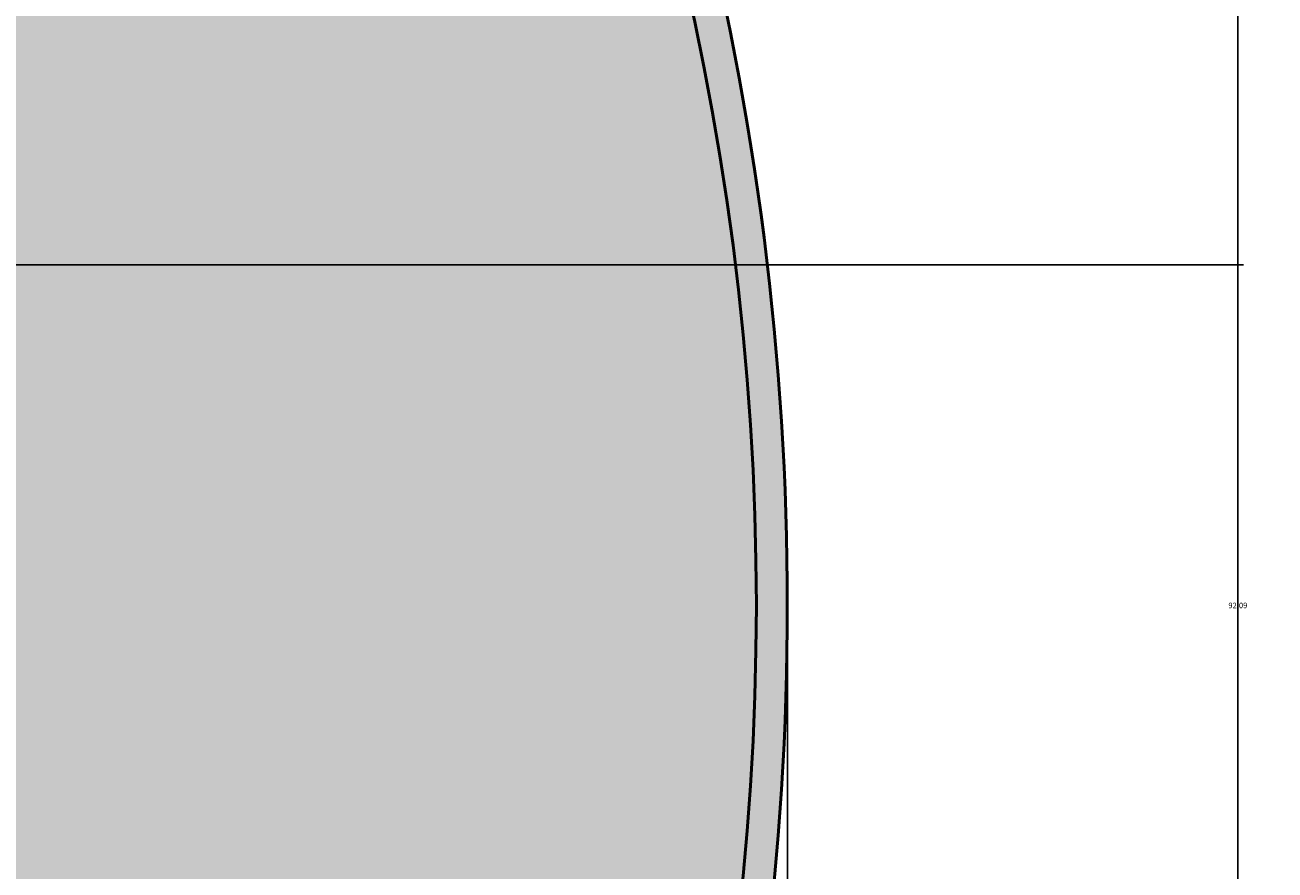
# Model space of a CAD drawing. Units: inches. Extents: x -12 to 334, y -10 to 186.
# Tile 73 of 77: x 257 to 297, y 83 to 111. Entities that reach past the tile are written whole.
import ezdxf

# ---------------------------------------------------------------- set-up
doc = ezdxf.new("R2010")
doc.units = ezdxf.units.IN
doc.header["$MEASUREMENT"] = 0
for name, color, linetype, lineweight in [('M-DIMS', 2, 'Continuous', 18), ('M-EQPM', 7, 'Continuous', 50), ('M-EQPM-PATT', 8, 'Continuous', 18)]:
    doc.layers.add(name, color=color, linetype=linetype, lineweight=lineweight)
doc.styles.get("Standard").update_dxf_attribs({"font": 'arial.ttf'})
doc.dimstyles.get("Standard").update_dxf_attribs({"dimtxt": 0.18, "dimasz": 0.18, "dimexe": 0.18, "dimexo": 0.0625, "dimgap": 0.09, "dimtad": 0, "dimtih": 1, "dimtoh": 1, "dimdec": 4, "dimzin": 0, "dimdsep": 46, "dimtxsty": 'Standard', "dimcen": 0.09, "dimadec": 0, "dimazin": 0, "dimtfac": 1, "dimtdec": 4, "dimtofl": 0, "dimtmove": 0, "dimatfit": 3, "dimfxl": 1, "dimtolj": 1, "dimtzin": 0, "dimarcsym": 0})

# ---------------------------------------------------------------- blocks, each defined once
blk = doc.blocks.new('*D1')
at = {"layer": 'Defpoints', "color": 0, "transparency": 16777216}
for p in [(281.426, 91.899), (3.376, 80.692), (281.426, 14.304)]:
    blk.add_point(p, dxfattribs=at)
at = {"layer": 'M-DIMS', "color": 0, "lineweight": -2, "transparency": 16777216}
for p, q in [((281.426, 91.836), (281.426, 14.124)), ((3.376, 80.629), (3.376, 14.124)), ((3.556, 14.304), (141.935, 14.304)), ((281.246, 14.304), (142.867, 14.304))]:
    blk.add_line(p, q, dxfattribs=at)
at = {"layer": 'M-DIMS', "color": 0, "transparency": 16777216}
for points in [[(3.556, 14.334), (3.556, 14.274), (3.376, 14.304)], [(281.246, 14.334), (281.246, 14.274), (281.426, 14.304)]]:
    blk.add_solid(points, dxfattribs=at)
at = {"layer": 'M-DIMS', "color": 0, "transparency": 16777216, "insert": (142.401, 14.304), "char_height": 0.18, "attachment_point": 5}
blk.add_mtext('\\A1;278.05', dxfattribs=at)
blk = doc.blocks.new('*D17')
at = {"layer": 'Defpoints', "color": 0, "transparency": 16777216}
for p in [(106.177, 102.896), (105.892, 56.321), (295.976, 56.321)]:
    blk.add_point(p, dxfattribs=at)
at = {"layer": 'M-DIMS', "color": 0, "lineweight": -2, "transparency": 16777216}
for p, q in [((106.24, 102.896), (296.156, 102.896)), ((295.976, 102.716), (295.976, 79.79)), ((295.976, 56.501), (295.976, 79.426)), ((105.954, 56.321), (296.156, 56.321))]:
    blk.add_line(p, q, dxfattribs=at)
at = {"layer": 'M-DIMS', "color": 0, "transparency": 16777216}
for points in [[(295.946, 102.716), (296.006, 102.716), (295.976, 102.896)], [(295.946, 56.501), (296.006, 56.501), (295.976, 56.321)]]:
    blk.add_solid(points, dxfattribs=at)
at = {"layer": 'M-DIMS', "color": 0, "transparency": 16777216, "insert": (295.976, 79.608), "char_height": 0.18, "attachment_point": 5}
blk.add_mtext('\\A1;46.575', dxfattribs=at)
blk = doc.blocks.new('*D24')
at = {"layer": 'Defpoints', "color": 0, "transparency": 16777216}
for p in [(269.381, 137.943), (269.381, 45.854), (295.976, 45.854)]:
    blk.add_point(p, dxfattribs=at)
at = {"layer": 'M-DIMS', "color": 0, "lineweight": -2, "transparency": 16777216}
for p, q in [((269.443, 137.943), (296.156, 137.943)), ((295.976, 137.763), (295.976, 92.081)), ((295.976, 46.034), (295.976, 91.717)), ((269.443, 45.854), (296.156, 45.854))]:
    blk.add_line(p, q, dxfattribs=at)
at = {"layer": 'M-DIMS', "color": 0, "transparency": 16777216}
for points in [[(295.946, 137.763), (296.006, 137.763), (295.976, 137.943)], [(295.946, 46.034), (296.006, 46.034), (295.976, 45.854)]]:
    blk.add_solid(points, dxfattribs=at)
at = {"layer": 'M-DIMS', "color": 0, "transparency": 16777216, "insert": (295.976, 91.899), "char_height": 0.18, "attachment_point": 5}
blk.add_mtext('\\A1;92.09', dxfattribs=at)
blk = doc.blocks.new('*D40')
at = {"layer": 'Defpoints', "color": 0, "transparency": 16777216}
for p in [(278.229, 116.208), (187.394, 91.899)]:
    blk.add_point(p, dxfattribs=at)
at = {"layer": 'M-DIMS', "color": 0, "lineweight": -2, "transparency": 16777216}
for p, q in [((332.73, 130.793), (278.403, 116.254)), ((187.304, 91.899), (187.484, 91.899)), ((187.394, 91.809), (187.394, 91.989))]:
    blk.add_line(p, q, dxfattribs=at)
at = {"layer": 'M-DIMS', "color": 0, "transparency": 16777216}
blk.add_solid([(278.395, 116.283), (278.411, 116.225), (278.229, 116.208)], dxfattribs=at)
at = {"layer": 'M-DIMS', "color": 0, "transparency": 16777216, "insert": (333.21, 130.793), "char_height": 0.18, "attachment_point": 5}
blk.add_mtext('\\A1;R94.03', dxfattribs=at)
blk = doc.blocks.new('*D41')
at = {"layer": 'Defpoints', "color": 0, "transparency": 16777216}
for p in [(190.169, 91.899), (277.343, 68.515)]:
    blk.add_point(p, dxfattribs=at)
at = {"layer": 'M-DIMS', "color": 0, "lineweight": -2, "transparency": 16777216}
for p, q in [((190.079, 91.899), (190.259, 91.899)), ((190.169, 91.809), (190.169, 91.989)), ((329.648, 54.485), (277.517, 68.469)), ((329.828, 54.485), (329.648, 54.485))]:
    blk.add_line(p, q, dxfattribs=at)
at = {"layer": 'M-DIMS', "color": 0, "transparency": 16777216}
blk.add_solid([(277.525, 68.498), (277.509, 68.44), (277.343, 68.515)], dxfattribs=at)
at = {"layer": 'M-DIMS', "color": 0, "transparency": 16777216, "insert": (330.307, 54.485), "char_height": 0.18, "attachment_point": 5}
blk.add_mtext('\\A1;R90.26', dxfattribs=at)

msp = doc.modelspace()

# ---------------------------------------------------------------- hatches: boundary and pattern name
at = {"layer": 'M-EQPM-PATT', "transparency": 33554556}
h = msp.add_hatch(color=256, dxfattribs=at)
h.set_gradient(color1=(248, 206, 179), color2=(248, 206, 179), tint=1)
h.paths.add_polyline_path([(179.7818, 136.8871), (126.9567, 136.8871), (106.1771, 100.8958), (171.5458, 100.8958)])
h.paths.add_polyline_path([(268.3808, 136.9435), (214.0166, 136.9435), (214.0166, 154.8345), (196.3421, 154.8345), (196.3421, 136.8871), (179.7818, 136.8871), (171.5458, 100.8958), (231.7758, 100.8958, -0.4142136), (251.9801, 80.6915), (279.7263, 80.6915, 0.1631825)])
at = {"layer": 'M-EQPM-PATT'}
h = msp.add_hatch(color=256, dxfattribs=at)
h.set_gradient(color1=(99, 100, 102), color2=(99, 100, 102), tint=1)
h.paths.add_polyline_path([(126.9567, 136.8871), (179.7818, 136.8871), (180.0106, 137.8871), (126.3793, 137.8871), (106.1771, 102.8958), (86.8879, 102.8958), (86.8879, 109.0583), (84.7229, 109.0583), (84.7229, 100.8958), (106.1771, 100.8958)])
h.paths.add_polyline_path([(196.3421, 152.8345), (195.3421, 152.8345), (195.3421, 137.8871), (180.0106, 137.8871), (179.7818, 136.8871), (196.3421, 136.8871)])
h.paths.add_polyline_path([(215.0166, 152.8345), (214.0166, 152.8345), (214.0166, 136.9435), (268.3808, 136.9435, -0.2673785), (268.3808, 46.8541), (249.3759, 46.8541), (249.8485, 45.8541), (269.3808, 45.8541, 0.2615891), (269.3808, 137.9435), (215.0166, 137.9435)])

# ---------------------------------------------------------------- linework, layer by layer
at = {"layer": 'M-EQPM'}
for centre, radius, start, end in [((187.3936, 91.8988), 94.032, 330.681071, 29.318929), ((190.1689, 91.8988), 90.256, 330.061028, 29.938972)]:
    msp.add_arc(centre, radius, start, end, dxfattribs=at)

# ---------------------------------------------------------------- dimensions: what is measured, and where the dimension line sits
at = {"layer": 'M-DIMS'}
for base, p1, p2, override, picture, middle in [((295.9756, 45.8541), (269.3808, 137.9435), (269.3808, 45.8541), {"dimdec": 2, "dimlfac": 1, "dimrnd": 0, "dimzin": 0, "dimdsep": 46, "dimlunit": 2}, '*D24', (295.9756, 91.8988)), ((295.9756, 56.3205), (106.1771, 102.8958), (105.8919, 56.3205), {"dimdec": 3, "dimlfac": 1, "dimrnd": 0, "dimzin": 0, "dimdsep": 46, "dimlunit": 2}, '*D17', (295.9756, 79.6082))]:
    dim = msp.add_linear_dim(base=base, p1=p1, p2=p2, angle=90, dimstyle='Standard', override=override, dxfattribs=at)
    dim.commit()
    dim.dimension.update_dxf_attribs({"geometry": picture, "text_midpoint": middle})
for center, mpoint, picture, middle in [((187.3936, 91.8988), (278.2291, 116.2078), '*D40', (332.7304, 130.7932)), ((190.1689, 91.8988), (277.3431, 68.5153), '*D41', (330.3074, 54.4851))]:
    dim = msp.add_radius_dim(center=center, mpoint=mpoint, dimstyle='Standard', override={"dimdec": 2, "dimlfac": 1, "dimrnd": 0, "dimzin": 0, "dimdsep": 46, "dimlunit": 2}, dxfattribs=at)
    dim.commit()
    dim.dimension.update_dxf_attribs({"geometry": picture, "text_midpoint": middle, "dimtype": 164})
dim = msp.add_linear_dim(base=(281.4256, 14.3041), p1=(3.3765, 80.6915), p2=(281.4256, 91.8988), dimstyle='Standard', override={"dimdec": 2, "dimlfac": 1, "dimrnd": 0, "dimzin": 0, "dimdsep": 46, "dimlunit": 2}, dxfattribs=at)
dim.commit()
dim.dimension.update_dxf_attribs({"geometry": '*D1', "text_midpoint": (142.401, 14.3041)})

doc.saveas('drawing.dxf')
